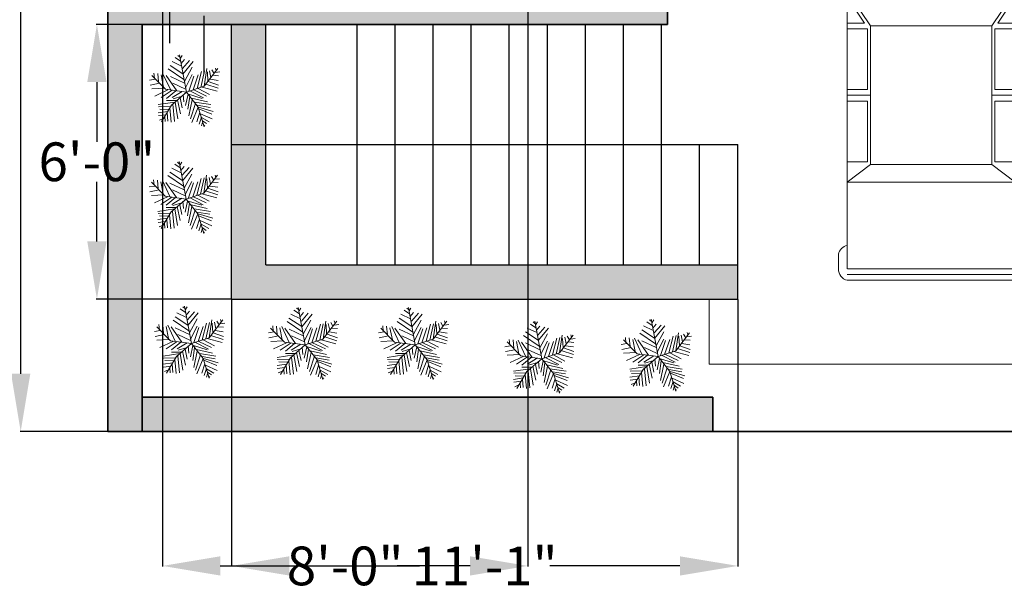
# Model space of a CAD drawing. Units: inches. Extents: x 19 to 15718, y 7 to 930.
# Tile 6 of 11: x 15243 to 15502, y 308 to 458. Entities that reach past the tile are written whole.
import ezdxf

# ---------------------------------------------------------------- set-up
doc = ezdxf.new("R2010")
doc.units = ezdxf.units.IN
doc.header["$MEASUREMENT"] = 0
for name, color, linetype, lineweight in [('A-ANNO-DIMS', 2, 'Continuous', 18), ('A-FLOR', 8, 'Continuous', 18), ('A-FLOR-STRS', 7, 'Continuous', 25), ('A-WALL', 7, 'Continuous', 35), ('C-PKNG-VEHC', 8, 'Continuous', 13), ('L-PLNT', 3, 'Continuous', 13)]:
    doc.layers.add(name, color=color, linetype=linetype, lineweight=lineweight)
doc.layers.add('A-WALL-PATT', color=18, linetype='Continuous', lineweight=13, true_color=0x000000)
doc.styles.get("Standard").update_dxf_attribs({"font": 'arial.ttf'})
doc.dimstyles.get("Standard").update_dxf_attribs({"dimtxt": 10.18, "dimasz": 15.18, "dimexe": 0.18, "dimexo": 0.0625, "dimgap": 0.09, "dimtad": 0, "dimtih": 1, "dimtoh": 1, "dimdec": 0, "dimzin": 0, "dimdsep": 46, "dimlunit": 3, "dimtxsty": 'Standard', "dimcen": 0.09, "dimadec": 0, "dimazin": 0, "dimtfac": 1, "dimtdec": 0, "dimtofl": 0, "dimtmove": 0, "dimatfit": 3, "dimfxl": 1, "dimtolj": 1, "dimtzin": 0, "dimarcsym": 0})

# ---------------------------------------------------------------- blocks, each defined once
blk = doc.blocks.new('*U13')
for p, q in [((-7.288, 39.707), (-21.778, 46.673)), ((-8.737, 47.138), (-17.069, 52.711)), ((-10.186, 53.64), (-13.084, 55.962)), ((0, 0), (-10.5, 57)), ((-9.099, 51.782), (-6.563, 55.962)), ((-7.65, 43.423), (-2.578, 49.46)), ((-5.839, 35.992), (4.667, 48.067)), ((-5.114, 27.632), (10.463, 46.673)), ((-3.665, 19.273), (-27.574, 35.527)), ((-5.114, 28.097), (-24.676, 40.636)), ((-2.941, 16.486), (8.652, 37.85)), ((16.259, 5.805), (23.142, 31.348)), ((22.055, 7.198), (27.489, 32.277)), ((27, 9), (48, 36)), ((27.127, 9.056), (31.112, 35.992)), ((31.836, 30.883), (32.561, 16.486)), ((35.096, 32.741), (37.27, 22.524)), ((38.719, 34.134), (41.979, 28.561)), ((43.791, 29.954), (51.036, 30.883)), ((44.153, 36.456), (45.239, 32.741)), ((-47.498, 19.737), (-55.83, 18.344)), ((-31.5, 4.5), (-52.5, 25.5)), ((-48.585, 21.131), (-49.309, 29.026)), ((-43.513, 28.561), (-42.427, 15.558)), ((-38.442, 26.239), (-34.819, 7.663)), ((-35.544, 28.097), (-24.314, 3.947)), ((-14.533, 2.09), (-30.834, 25.31)), ((-24.314, 23.917), (-2.941, 13.7)), ((-1.129, 6.734), (9.014, 26.704)), ((3.942, 1.625), (11.187, 24.381)), ((10.101, 3.483), (17.708, 26.239)), ((33.285, 16.486), (48.862, 10.913)), ((36.183, 19.737), (48.137, 17.88)), ((40.53, 25.775), (48.862, 24.846)), ((-40.615, 13.7), (-55.105, 10.913)), ((-33.37, 6.269), (-52.207, 5.34)), ((-28.299, 3.483), (-47.86, -5.805)), ((-21.416, 3.018), (-38.079, -8.128)), ((0, 0), (-31.5, 4.5)), ((-15.982, 2.09), (-30.11, -9.521)), ((0, 0), (-22.5, -19.5)), ((-6.563, 1.161), (-21.416, -8.128)), ((-20.691, 13.7), (-1.129, 4.876)), ((0, 0), (27, 9)), ((0, 0), (18, -22.5)), ((6.478, 1.625), (26.04, -8.592)), ((11.187, 3.483), (30.749, -5.805)), ((18.07, 5.805), (35.096, -3.483)), ((24.229, 7.663), (46.688, 1.625)), ((29.662, 12.307), (48.137, 6.269)), ((-15.257, -12.772), (-30.11, -12.772)), ((-6.563, -5.805), (-19.967, -9.985)), ((-13.446, -11.378), (-8.737, -32.741)), ((-9.461, -8.592), (-6.201, -23.453)), ((-4.752, -3.483), (-3.665, -14.629)), ((2.493, -3.019), (-1.491, -20.202)), ((1.769, -2.555), (24.229, -9.521)), ((5.029, -6.27), (2.131, -25.775)), ((9.014, -11.378), (3.58, -35.992)), ((7.565, -9.056), (32.198, -14.629)), ((-17.431, -15.094), (-42.789, -18.809)), ((-28.299, -29.026), (-42.789, -31.348)), ((-24.314, -21.596), (-42.427, -22.06)), ((-26.849, -26.24), (-40.253, -25.775)), ((-22.5, -19.5), (-37.5, -45)), ((-25.038, -23.918), (-22.865, -45.281)), ((-20.691, -18.345), (-17.793, -44.352)), ((-17.069, -15.094), (-12.721, -40.172)), ((14.085, -16.951), (6.478, -40.172)), ((18.07, -22.524), (8.289, -45.745)), ((12.274, -15.094), (36.907, -18.809)), ((16.259, -19.738), (36.183, -22.989)), ((18, -22.5), (27, -52.5)), ((18.433, -22.524), (40.53, -29.026)), ((19.157, -25.311), (38.719, -33.206)), ((-30.834, -34.135), (-42.427, -35.528)), ((-34.457, -39.708), (-40.978, -42.494)), ((-32.646, -36.921), (-31.921, -44.352)), ((-29.023, -30.884), (-27.936, -43.887)), ((20.244, -30.419), (15.897, -44.816)), ((22.78, -37.85), (19.519, -48.532)), ((21.331, -32.741), (39.081, -40.636)), ((22.78, -38.314), (34.372, -44.816)), ((24.591, -43.423), (30.749, -47.603)), ((24.591, -45.745), (23.142, -50.854)), ((26.764, -49.925), (28.213, -50.854))]:
    blk.add_line(p, q)
blk = doc.blocks.new('*U14')
for p, q in [((5.44, 42.31), (12.12, 42.31)), ((189.69, 42.31), (183.01, 42.31)), ((0.1, -0.41), (0.1, 38.35)), ((2.77, -0.41), (2.77, 38.31)), ((5.44, -0.41), (5.44, 38.24)), ((5.45, 38.31), (16.12, 38.31)), ((16.12, 38.31), (180.34, 38.31)), ((61.52, -0.41), (61.52, 38.31)), ((61.52, 38.31), (77.54, 27.62)), ((64.19, 38.31), (76.2, 30.29)), ((76.2, 30.29), (76.2, 38.31)), ((78.87, 38.31), (78.87, 28.96)), ((106.91, 28.96), (106.91, 38.31)), ((109.58, 27.62), (109.58, 38.31)), ((112.25, 38.31), (112.25, 28.96)), ((140.29, 28.96), (140.29, 38.31)), ((141.62, 27.62), (149.64, 38.31)), ((149.64, -0.41), (149.64, 38.31)), ((189.69, 38.31), (179.01, 38.31)), ((189.69, -0.41), (189.69, 38.24)), ((192.36, -0.41), (192.36, 38.31)), ((195.03, -0.41), (195.03, 38.35)), ((77.54, 27.62), (141.62, 27.62)), ((77.54, -0.41), (77.54, 27.62)), ((78.87, 28.96), (106.91, 28.96)), ((112.25, 28.96), (140.29, 28.96)), ((141.62, -0.41), (141.62, 27.62)), ((5.44, 7.6), (61.52, 15.61)), ((0.1, -0.42), (0.1, -39.18)), ((2.77, -0.41), (2.77, -39.13)), ((5.44, -0.42), (5.44, -39.07)), ((61.52, -0.41), (61.52, -39.13)), ((77.54, -0.41), (77.54, -28.45)), ((141.62, -0.41), (141.62, -28.45)), ((149.64, -0.41), (149.64, -39.13)), ((189.69, -0.42), (189.69, -39.07)), ((192.36, -0.41), (192.36, -39.13)), ((195.03, -0.42), (195.03, -39.18)), ((5.44, -8.42), (61.52, -16.43)), ((61.52, -39.13), (77.54, -28.45)), ((64.19, -39.13), (76.2, -31.12)), ((76.2, -31.12), (76.2, -39.13)), ((77.54, -28.45), (141.62, -28.45)), ((78.87, -39.13), (78.87, -29.79)), ((78.87, -29.79), (106.91, -29.79)), ((106.91, -29.79), (106.91, -39.13)), ((109.58, -28.45), (109.58, -39.13)), ((112.25, -29.79), (140.29, -29.79)), ((112.25, -39.13), (112.25, -29.79)), ((140.29, -29.79), (140.29, -39.13)), ((141.62, -28.45), (149.64, -39.13)), ((5.45, -39.13), (16.12, -39.13)), ((16.12, -39.13), (180.34, -39.13)), ((189.69, -39.13), (179.01, -39.13)), ((5.44, -43.14), (12.12, -43.14)), ((189.69, -43.14), (183.01, -43.14))]:
    blk.add_line(p, q)
for centre, radius, start, end in [((5.06, 37.26), 5.06, 85.6455, 168.0943), ((11.45, 37.64), 4.72, 8.1301, 81.87), ((183.68, 37.64), 4.72, 98.13, 171.8699), ((190.07, 37.26), 5.06, 11.9057, 94.3545), ((5.06, -38.09), 5.06, 191.9057, 274.3545), ((11.45, -38.46), 4.72, 278.13, 351.8699), ((183.68, -38.46), 4.72, 188.1301, 261.87), ((190.07, -38.09), 5.06, 265.6455, 348.0943)]:
    blk.add_arc(centre, radius, start, end)
blk = doc.blocks.new('*D17')
at = {"layer": 'A-ANNO-DIMS', "color": 0, "lineweight": -2, "transparency": 16777216}
for p, q in [((15266.62, 830.27), (15243.58, 830.27)), ((15243.76, 815.09), (15243.76, 595.52)), ((15243.76, 365.38), (15243.76, 584.95)), ((15266.62, 350.2), (15243.58, 350.2))]:
    blk.add_line(p, q, dxfattribs=at)
at = {"layer": 'A-ANNO-DIMS', "color": 0, "transparency": 16777216}
for points in [[(15241.23, 815.09), (15246.29, 815.09), (15243.76, 830.27)], [(15241.23, 365.38), (15246.29, 365.38), (15243.76, 350.2)]]:
    blk.add_solid(points, dxfattribs=at)
at = {"layer": 'Defpoints', "color": 0, "transparency": 16777216}
for p in [(15266.68, 830.27), (15243.76, 350.2), (15266.68, 350.2)]:
    blk.add_point(p, dxfattribs=at)
at = {"layer": 'A-ANNO-DIMS', "color": 0, "transparency": 16777216, "insert": (15243.76, 590.24), "char_height": 10.18, "attachment_point": 5}
blk.add_mtext("\\A1;40'", dxfattribs=at)
blk = doc.blocks.new('*D60')
at = {"layer": 'A-ANNO-DIMS', "color": 0, "lineweight": -2, "transparency": 16777216}
for p, q in [((15125.78, 484.16), (15125.78, 483.21)), ((15131.32, 484.16), (15131.32, 483.21)), ((15110.6, 483.39), (15095.42, 483.39)), ((15146.5, 483.39), (15161.68, 483.39))]:
    blk.add_line(p, q, dxfattribs=at)
at = {"layer": 'A-ANNO-DIMS', "color": 0, "transparency": 16777216}
for points in [[(15110.6, 485.92), (15110.6, 480.86), (15125.78, 483.39)], [(15146.5, 485.92), (15146.5, 480.86), (15131.32, 483.39)]]:
    blk.add_solid(points, dxfattribs=at)
at = {"layer": 'Defpoints', "color": 0, "transparency": 16777216}
for p in [(15125.78, 484.23), (15131.32, 484.23), (15131.32, 483.39)]:
    blk.add_point(p, dxfattribs=at)
at = {"layer": 'A-ANNO-DIMS', "color": 0, "transparency": 16777216, "insert": (15253.56, 483.39), "char_height": 10.18, "attachment_point": 5}
blk.add_mtext('\\A1;GAS BURNER 0\'-5 1/2" TYP.', dxfattribs=at)
blk = doc.blocks.new('*D62')
at = {"layer": 'A-ANNO-DIMS', "color": 0, "lineweight": -2, "transparency": 16777216}
for p, q in [((15269.83, 473.76), (15254.65, 473.76)), ((15285.01, 474.6), (15285.01, 473.58)), ((15291.01, 474.6), (15291.01, 473.58)), ((15306.19, 473.76), (15321.37, 473.76))]:
    blk.add_line(p, q, dxfattribs=at)
at = {"layer": 'A-ANNO-DIMS', "color": 0, "transparency": 16777216}
for points in [[(15269.83, 476.29), (15269.83, 471.23), (15285.01, 473.76)], [(15306.19, 476.29), (15306.19, 471.23), (15291.01, 473.76)]]:
    blk.add_solid(points, dxfattribs=at)
at = {"layer": 'Defpoints', "color": 0, "transparency": 16777216}
for p in [(15285.01, 474.66), (15291.01, 474.66), (15291.01, 473.76)]:
    blk.add_point(p, dxfattribs=at)
at = {"layer": 'A-ANNO-DIMS', "color": 0, "transparency": 16777216, "insert": (15413.32, 473.76), "char_height": 10.18, "attachment_point": 5}
blk.add_mtext('\\A1;SMALL ELEMENT 0\'-6" TYP.', dxfattribs=at)
blk = doc.blocks.new('*D63')
at = {"layer": 'A-ANNO-DIMS', "color": 0, "lineweight": -2, "transparency": 16777216}
for p, q in [((15291.91, 495.84), (15291.91, 511.02)), ((15291.91, 511.02), (15307.09, 511.02)), ((15291.07, 480.66), (15292.09, 480.66)), ((15291.07, 474.66), (15292.09, 474.66)), ((15291.91, 459.48), (15291.91, 444.3))]:
    blk.add_line(p, q, dxfattribs=at)
at = {"layer": 'A-ANNO-DIMS', "color": 0, "transparency": 16777216}
for points in [[(15289.38, 495.84), (15294.44, 495.84), (15291.91, 480.66)], [(15289.38, 459.48), (15294.44, 459.48), (15291.91, 474.66)]]:
    blk.add_solid(points, dxfattribs=at)
at = {"layer": 'Defpoints', "color": 0, "transparency": 16777216}
for p in [(15291.01, 480.66), (15291.91, 480.66), (15291.01, 474.66)]:
    blk.add_point(p, dxfattribs=at)
at = {"layer": 'A-ANNO-DIMS', "color": 0, "transparency": 16777216, "insert": (15338.21, 511.02), "char_height": 10.18, "attachment_point": 5}
blk.add_mtext('\\A1;0\'-6" TYP.', dxfattribs=at)
blk = doc.blocks.new('*D65')
at = {"layer": 'A-ANNO-DIMS', "color": 0, "lineweight": -2, "transparency": 16777216}
for p, q in [((15282.81, 505.84), (15282.81, 521.02)), ((15282.81, 521.02), (15297.99, 521.02)), ((15283.95, 490.66), (15282.63, 490.66)), ((15283.95, 482.66), (15282.63, 482.66)), ((15282.81, 467.48), (15282.81, 452.3))]:
    blk.add_line(p, q, dxfattribs=at)
at = {"layer": 'A-ANNO-DIMS', "color": 0, "transparency": 16777216}
for points in [[(15280.28, 505.84), (15285.34, 505.84), (15282.81, 490.66)], [(15280.28, 467.48), (15285.34, 467.48), (15282.81, 482.66)]]:
    blk.add_solid(points, dxfattribs=at)
at = {"layer": 'Defpoints', "color": 0, "transparency": 16777216}
for p in [(15282.81, 490.66), (15284.01, 490.66), (15284.01, 482.66)]:
    blk.add_point(p, dxfattribs=at)
at = {"layer": 'A-ANNO-DIMS', "color": 0, "transparency": 16777216, "insert": (15329.11, 521.02), "char_height": 10.18, "attachment_point": 5}
blk.add_mtext('\\A1;0\'-8" TYP.', dxfattribs=at)
blk = doc.blocks.new('*D76')
at = {"layer": 'A-ANNO-DIMS', "color": 0, "lineweight": -2, "transparency": 16777216}
for p, q in [((15299.13, 384.91), (15299.13, 314.67)), ((15432.13, 384.91), (15432.13, 314.67)), ((15314.31, 314.85), (15348.53, 314.85)), ((15416.95, 314.85), (15382.73, 314.85))]:
    blk.add_line(p, q, dxfattribs=at)
at = {"layer": 'A-ANNO-DIMS', "color": 0, "transparency": 16777216}
for points in [[(15314.31, 317.38), (15314.31, 312.32), (15299.13, 314.85)], [(15416.95, 317.38), (15416.95, 312.32), (15432.13, 314.85)]]:
    blk.add_solid(points, dxfattribs=at)
at = {"layer": 'Defpoints', "color": 0, "transparency": 16777216}
for p in [(15299.13, 384.97), (15432.13, 384.97), (15432.13, 314.85)]:
    blk.add_point(p, dxfattribs=at)
at = {"layer": 'A-ANNO-DIMS', "color": 0, "transparency": 16777216, "insert": (15365.63, 314.85), "char_height": 10.18, "attachment_point": 5}
blk.add_mtext('\\A1;11\'-1"', dxfattribs=at)
blk = doc.blocks.new('*D77')
at = {"layer": 'A-ANNO-DIMS', "color": 0, "lineweight": -2, "transparency": 16777216}
for p, q in [((15299.066506, 457.203955), (15263.599006, 457.203955)), ((15263.779006, 442.023955), (15263.779006, 426.374109)), ((15263.779006, 400.148997), (15263.779006, 415.798843)), ((15299.066506, 384.968997), (15263.599006, 384.968997))]:
    blk.add_line(p, q, dxfattribs=at)
at = {"layer": 'A-ANNO-DIMS', "color": 0, "transparency": 16777216}
for points in [[(15261.249006, 442.023955), (15266.309006, 442.023955), (15263.779006, 457.203955)], [(15261.249006, 400.148997), (15266.309006, 400.148997), (15263.779006, 384.968997)]]:
    blk.add_solid(points, dxfattribs=at)
at = {"layer": 'Defpoints', "color": 0, "transparency": 16777216}
for p in [(15263.779006, 457.203955), (15299.129006, 457.203955), (15299.129006, 384.968997)]:
    blk.add_point(p, dxfattribs=at)
at = {"layer": 'A-ANNO-DIMS', "color": 0, "transparency": 16777216, "insert": (15263.779006, 421.086476), "char_height": 10.18, "attachment_point": 5}
blk.add_mtext('\\A1;6\'-0"', dxfattribs=at)
blk = doc.blocks.new('*D80')
at = {"layer": 'A-ANNO-DIMS', "color": 0, "lineweight": -2, "transparency": 16777216}
for p, q in [((15602.030581, 511.142303), (15602.030581, 526.322303)), ((15181.899116, 495.962303), (15602.210581, 495.962303)), ((15181.899116, 469.995573), (15602.210581, 469.995573)), ((15602.030581, 454.815573), (15602.030581, 439.635573))]:
    blk.add_line(p, q, dxfattribs=at)
at = {"layer": 'A-ANNO-DIMS', "color": 0, "transparency": 16777216}
for points in [[(15599.500581, 511.142303), (15604.560581, 511.142303), (15602.030581, 495.962303)], [(15599.500581, 454.815573), (15604.560581, 454.815573), (15602.030581, 469.995573)]]:
    blk.add_solid(points, dxfattribs=at)
at = {"layer": 'Defpoints', "color": 0, "transparency": 16777216}
for p in [(15181.836616, 495.962303), (15602.030581, 495.962303), (15181.836616, 469.995573)]:
    blk.add_point(p, dxfattribs=at)
at = {"layer": 'A-ANNO-DIMS', "color": 0, "transparency": 16777216, "insert": (15602.030581, 482.978938), "char_height": 10.18, "attachment_point": 5}
blk.add_mtext('\\A1;2\'-2"', dxfattribs=at)
blk = doc.blocks.new('*D81')
at = {"layer": 'A-ANNO-DIMS', "color": 0, "lineweight": -2, "transparency": 16777216}
for p, q in [((15281.01, 559.14), (15281.01, 314.67)), ((15377.01, 559.14), (15377.01, 314.67)), ((15296.19, 314.85), (15315.38, 314.85)), ((15361.83, 314.85), (15342.64, 314.85))]:
    blk.add_line(p, q, dxfattribs=at)
at = {"layer": 'A-ANNO-DIMS', "color": 0, "transparency": 16777216}
for points in [[(15296.19, 317.38), (15296.19, 312.32), (15281.01, 314.85)], [(15361.83, 317.38), (15361.83, 312.32), (15377.01, 314.85)]]:
    blk.add_solid(points, dxfattribs=at)
at = {"layer": 'Defpoints', "color": 0, "transparency": 16777216}
for p in [(15281.01, 559.2), (15377.01, 559.2), (15377.01, 314.85)]:
    blk.add_point(p, dxfattribs=at)
at = {"layer": 'A-ANNO-DIMS', "color": 0, "transparency": 16777216, "insert": (15329.01, 314.85), "char_height": 10.18, "attachment_point": 5}
blk.add_mtext('\\A1;8\'-0"', dxfattribs=at)

msp = doc.modelspace()

# ---------------------------------------------------------------- hatches: boundary and pattern name
at = {"layer": 'A-WALL-PATT'}
h = msp.add_hatch(color=256, dxfattribs=at)
h.dxf.hatch_style = 1
h.paths.add_polyline_path([(15190.84, 837), (14890.84, 837), (14890.84, 357), (14899.84, 357), (14899.84, 366), (14899.84, 528), (14904.84, 528), (14904.84, 534), (14899.84, 534), (14899.84, 698), (15004.84, 698), (15004.84, 701, -0.014283), (15004.84, 703), (15004.84, 704), (14899.84, 704), (14899.84, 828), (14987.26, 828), (15043.84, 828), (15049.84, 828), (15075.84, 828), (15081.84, 828), (15181.84, 828), (15181.84, 780), (15114.84, 780), (15114.84, 779, -0.017236), (15114.84, 777), (15114.84, 774), (15181.84, 774), (15181.84, 654), (15181.84, 648), (15181.84, 596), (15190.84, 596)])
h.paths.add_polyline_path([(15190.84, 590), (15181.84, 590), (15181.84, 470), (15181.84, 464), (15181.84, 361.43), (14991.9, 361.43), (14991.5, 357), (15190.84, 357)], flags=0)
h.paths.add_polyline_path([(15152.29, 608), (15146.29, 608), (15146.29, 596), (15049.84, 596), (15049.84, 590), (15152.29, 590)], flags=17)
h.paths.add_polyline_path([(15049.84, 615), (15048.84, 615, -0.017236), (15046.84, 615), (15043.84, 615), (15043.84, 596), (15049.84, 596)], flags=17)
edge = h.paths.add_edge_path(flags=17)
edge.add_line((15152.29, 654), (15049.84, 654))
edge.add_line((15049.84, 654), (15043.84, 654))
edge.add_line((15043.84, 654), (15043.84, 648))
edge.add_line((15043.84, 648), (15049.84, 648))
edge.add_line((15049.84, 648), (15075.84, 648))
edge.add_line((15075.84, 648), (15081.84, 648))
edge.add_line((15081.84, 648), (15117.26, 648))
edge.add_spline(control_points=[(15117.26, 648), (15117.59, 648.02), (15117.94, 648.03), (15118.71, 648.04), (15119.15, 648.02), (15119.59, 648)], knot_values=[1.499122, 1.499122, 1.499122, 1.499122, 1.618335, 1.618335, 1.770388, 1.770388, 1.770388, 1.770388], degree=3, periodic=0)
edge.add_spline(control_points=[(15127.99, 642.93), (15128, 643.28), (15127.95, 643.62), (15127.73, 644.26), (15127.57, 644.57), (15127.16, 645.13), (15126.92, 645.39), (15126.04, 646.16), (15125.28, 646.6), (15123.53, 647.31), (15122.55, 647.59), (15120.88, 647.88), (15120.24, 647.95), (15119.59, 648)], knot_values=[0, 0, 0, 0, 0.172075, 0.172075, 0.344149, 0.344149, 0.516224, 0.516224, 0.894541, 0.894541, 1.272858, 1.272858, 1.499122, 1.499122, 1.499122, 1.499122], degree=3, periodic=0)
edge.add_line((15119.59, 648), (15146.29, 648))
edge.add_line((15146.29, 648), (15146.29, 636))
edge.add_line((15146.29, 636), (15152.29, 636))
edge.add_line((15152.29, 636), (15152.29, 654))
h.paths.add_polyline_path([(15132.35, 430.4), (15123.35, 430.4), (15123.35, 396.8), (15027.77, 396.8), (15027.77, 387.8), (15132.35, 387.8)], flags=17)
h.paths.add_polyline_path([(15132.35, 464), (15123.35, 464), (15123.35, 430.4), (15132.35, 430.4)], flags=17)
h.paths.add_polyline_path([(15275.68, 583.59), (15276.07, 583.2), (15276.65, 583.2), (15280.6, 587.16), (15278.55, 589.2), (15275.68, 589.2), (15275.68, 601.2), (15266.68, 601.2), (15266.68, 350.2), (15275.68, 350.2), (15275.68, 359.2), (15275.68, 457.2), (15413.68, 457.2), (15413.68, 471.04), (15407.68, 471.04), (15407.68, 463.2), (15275.68, 463.2)])
h = msp.add_hatch(color=256, dxfattribs=at)
h.dxf.hatch_style = 1
h.paths.add_polyline_path([(15566.68, 830.2), (15266.68, 830.2), (15266.68, 629.2), (15275.68, 629.2), (15275.68, 641.2), (15301.68, 641.2), (15301.68, 589.2), (15275.68, 589.2), (15275.68, 601.2), (15266.68, 601.2), (15266.68, 350.2), (15275.68, 350.2), (15275.68, 359.2), (15275.68, 457.2), (15413.68, 457.2), (15413.68, 471.04), (15407.68, 471.04), (15407.68, 463.2), (15275.68, 463.2), (15275.68, 583.59), (15276.07, 583.2), (15276.65, 583.2), (15277.42, 583.97), (15276.36, 585.03), (15279.54, 588.22), (15280.6, 587.16), (15281.66, 588.22), (15282.72, 587.16), (15283.78, 588.22), (15284.85, 587.16), (15285.91, 588.22), (15286.97, 587.16), (15288.03, 588.22), (15289.09, 587.16), (15290.15, 588.22), (15291.21, 587.16), (15292.27, 588.22), (15293.33, 587.16), (15294.39, 588.22), (15295.45, 587.16), (15296.51, 588.22), (15297.57, 587.16), (15298.63, 588.22), (15299.69, 587.16), (15300.76, 588.22), (15301.82, 587.16), (15302.88, 588.22), (15303.94, 587.16), (15305, 588.22), (15306.06, 587.16), (15307.68, 588.78), (15307.68, 641.2), (15407.68, 641.2), (15413.68, 641.2), (15413.68, 647.2), (15407.68, 647.2), (15275.68, 647.2), (15275.68, 767.2), (15336.68, 767.2), (15336.68, 773.2), (15275.68, 773.2), (15275.68, 821.2), (15375.68, 821.2), (15381.68, 821.2), (15407.68, 821.2), (15413.68, 821.2), (15557.68, 821.2), (15557.68, 697.2), (15452.68, 697.2), (15452.68, 696.2, -0.014283), (15452.68, 694.2), (15452.68, 691.2), (15557.68, 691.2), (15557.68, 527.2), (15557.68, 521.2), (15557.68, 359.2), (15557.68, 350.2), (15566.68, 350.2)])
h.paths.add_polyline_path([(15416.63, 527.2), (15413.68, 527.2), (15407.68, 527.2), (15407.68, 521.04), (15413.68, 521.04), (15413.68, 521.2), (15416.63, 521.2)], flags=17)
h.paths.add_polyline_path([(15432.13, 393.97), (15308.13, 393.97), (15308.13, 425.59), (15299.13, 425.59), (15299.13, 384.97), (15432.13, 384.97)], flags=17)
h.paths.add_polyline_path([(15308.13, 457.2), (15299.13, 457.2), (15299.13, 425.59), (15308.13, 425.59)], flags=17)
h.paths.add_polyline_path([(15425.57, 359.2), (15275.68, 359.2), (15275.68, 350.2), (15425.57, 350.2)], flags=17)
h.paths.add_polyline_path([(15413.68, 797.2), (15407.68, 797.2), (15407.68, 773.2), (15381.68, 773.2), (15381.68, 797.2), (15375.68, 797.2), (15375.68, 773.2), (15375.68, 767.2), (15407.68, 767.2), (15407.68, 686.2), (15408.68, 686.2, -0.014283), (15410.68, 686.2), (15413.68, 686.2), (15413.68, 691.2), (15413.68, 697.2)], flags=17)
h.paths.add_polyline_path([(15413.68, 608.2), (15410.68, 608.2, -0.017236), (15408.68, 608.2), (15407.68, 608.2), (15407.68, 589.2), (15388.16, 589.2, -0.313626), (15386.75, 588.23), (15381.37, 588.23), (15380.3, 587.16), (15381.37, 586.1), (15380.3, 585.03), (15382.14, 583.2), (15407.68, 583.2), (15413.68, 583.2)], flags=17)

# ---------------------------------------------------------------- linework, layer by layer
at = {"layer": 'A-FLOR'}
for p, q in [((15424.65, 367.9), (15424.65, 384.97)), ((15557.68, 367.9), (15424.65, 367.9))]:
    msp.add_line(p, q, dxfattribs=at)
at = {"layer": 'A-FLOR-STRS'}
for p, q in [((15299.13, 384.97), (15299.13, 457.2)), ((15299.13, 393.97), (15299.13, 457.2)), ((15308.13, 393.97), (15308.13, 457.2)), ((15332.13, 393.97), (15332.13, 457.2)), ((15342.13, 393.97), (15342.13, 457.2)), ((15352.13, 393.97), (15352.13, 457.2)), ((15362.13, 393.97), (15362.13, 457.2)), ((15372.13, 393.97), (15372.13, 457.2)), ((15382.13, 393.97), (15382.13, 457.2)), ((15382.13, 393.97), (15382.13, 457.2)), ((15392.13, 393.97), (15392.13, 457.2)), ((15402.13, 393.97), (15402.13, 457.2)), ((15412.13, 393.97), (15412.13, 457.2)), ((15299.13, 425.59), (15432.13, 425.59)), ((15422.13, 393.97), (15422.13, 425.59)), ((15432.13, 384.97), (15432.13, 425.59)), ((15308.13, 393.97), (15432.13, 393.97)), ((15299.13, 384.97), (15432.13, 384.97))]:
    msp.add_line(p, q, dxfattribs=at)
at = {"layer": 'A-WALL'}
for p, q in [((15266.68, 350.2), (15266.68, 830.2)), ((15413.68, 521.2), (15413.68, 457.2)), ((15275.68, 359.2), (15275.68, 457.2)), ((15275.68, 457.2), (15413.68, 457.2)), ((15425.57, 359.2), (15275.68, 359.2)), ((15275.68, 359.2), (15275.68, 350.2)), ((15425.57, 359.2), (15425.57, 350.2)), ((15425.57, 350.2), (15266.68, 350.2)), ((15425.57, 350.2), (15557.68, 350.2))]:
    msp.add_line(p, q, dxfattribs=at)

# ---------------------------------------------------------------- block references
at = {"layer": 'C-PKNG-VEHC', "xscale": 0.5691226359303588, "yscale": 0.5691226359303588, "zscale": 0.5691226359303588, "rotation": 270}
msp.add_blockref('*U14', (15483.19, 500.93), dxfattribs=at)
at = {"layer": 'L-PLNT', "xscale": 0.1731210991633179, "yscale": 0.1731210991633179, "zscale": 0.1731210991633179}
for p in [(15287.28, 439.37), (15287.19, 411.3), (15288.59, 373.28), (15318.5, 372.93), (15347.43, 372.93), (15380.63, 369.31), (15411.19, 369.86)]:
    msp.add_blockref('*U13', p, dxfattribs=at)

# ---------------------------------------------------------------- dimensions: what is measured, and where the dimension line sits
at = {"layer": 'A-ANNO-DIMS'}
for base, p1, p2, override, picture, middle in [((15243.76, 350.2), (15266.68, 830.27), (15266.68, 350.2), {"dimclrd": 0, "dimclre": 0, "dimclrt": 0}, '*D17', (15243.76, 590.24)), ((15602.03, 495.96), (15181.84, 470), (15181.84, 495.96), {"dimdec": 1, "dimlfac": 1, "dimrnd": 0, "dimzin": 1, "dimdsep": 46, "dimlunit": 4, "dimfrac": 2}, '*D80', (15602.03, 482.98)), ((15263.78, 457.2), (15299.13, 384.97), (15299.13, 457.2), {"dimdec": 1, "dimlfac": 1, "dimrnd": 0, "dimzin": 1, "dimdsep": 46, "dimlunit": 4, "dimfrac": 2}, '*D77', (15263.78, 421.09))]:
    dim = msp.add_linear_dim(base=base, p1=p1, p2=p2, angle=90, dimstyle='Standard', override=override, dxfattribs=at)
    dim.commit()
    dim.dimension.update_dxf_attribs({"geometry": picture, "text_midpoint": middle})
for base, p1, p2, picture, middle in [((15377.01, 314.85), (15281.01, 559.2), (15377.01, 559.2), '*D81', (15329.01, 314.85)), ((15432.13, 314.85), (15299.13, 384.97), (15432.13, 384.97), '*D76', (15365.63, 314.85))]:
    dim = msp.add_linear_dim(base=base, p1=p1, p2=p2, dimstyle='Standard', override={"dimdec": 1, "dimlfac": 1, "dimrnd": 0, "dimzin": 1, "dimdsep": 46, "dimlunit": 4, "dimfrac": 2}, dxfattribs=at)
    dim.commit()
    dim.dimension.update_dxf_attribs({"geometry": picture, "text_midpoint": middle})
for base, p1, p2, picture, middle in [((15282.81, 490.66), (15284.01, 482.66), (15284.01, 490.66), '*D65', (15329.11, 521.02)), ((15291.91, 480.66), (15291.01, 474.66), (15291.01, 480.66), '*D63', (15338.21, 511.02))]:
    dim = msp.add_linear_dim(base=base, p1=p1, p2=p2, angle=90, text='<> TYP.', dimstyle='Standard', override={"dimdec": 1, "dimlfac": 1, "dimrnd": 0, "dimzin": 1, "dimdsep": 46, "dimlunit": 4, "dimfrac": 2}, dxfattribs=at)
    dim.commit()
    dim.dimension.update_dxf_attribs({"geometry": picture, "text_midpoint": middle})
for base, p1, p2, text, picture, middle in [((15131.32, 483.39), (15125.78, 484.23), (15131.32, 484.23), 'GAS BURNER <> TYP.', '*D60', (15253.56, 483.39)), ((15291.01, 473.76), (15285.01, 474.66), (15291.01, 474.66), 'SMALL ELEMENT <> TYP.', '*D62', (15413.32, 473.76))]:
    dim = msp.add_linear_dim(base=base, p1=p1, p2=p2, text=text, dimstyle='Standard', override={"dimdec": 1, "dimlfac": 1, "dimrnd": 0, "dimzin": 1, "dimdsep": 46, "dimlunit": 4, "dimfrac": 2}, dxfattribs=at)
    dim.commit()
    dim.dimension.update_dxf_attribs({"geometry": picture, "text_midpoint": middle})

doc.saveas('drawing.dxf')
